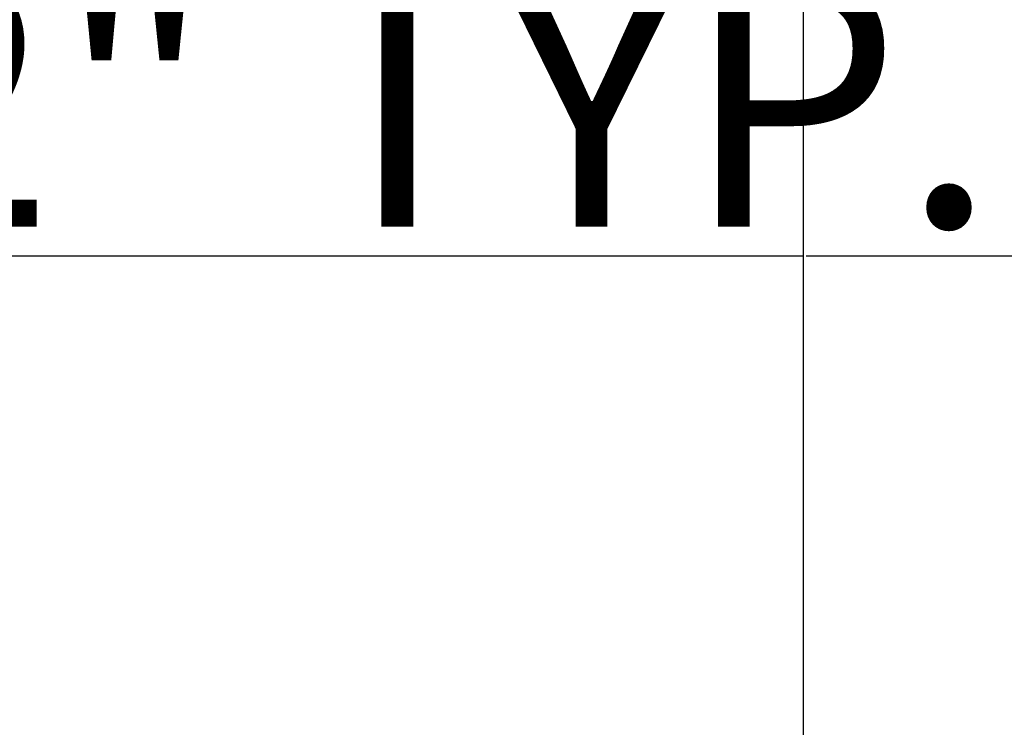
# Model space of a CAD drawing. Units: inches. Extents: x 2278 to 7495, y -71 to 1198.
# Tile 29 of 44: x 5127 to 5150, y 107 to 124. Entities that reach past the tile are written whole.
import ezdxf

# ---------------------------------------------------------------- set-up
doc = ezdxf.new("R2010")
doc.units = ezdxf.units.IN
doc.header["$MEASUREMENT"] = 0
doc.layers.add('A-ANNO-DIMS', color=2, linetype='Continuous', lineweight=18)
doc.layers.add('A-ELEV', color=7, linetype='Continuous', lineweight=25)
doc.styles.get("Standard").update_dxf_attribs({"font": 'arial.ttf'})
doc.dimstyles.get("Standard").update_dxf_attribs({"dimtxt": 6, "dimasz": 3, "dimexe": 0.18, "dimexo": 0.0625, "dimgap": 0.09, "dimtad": 0, "dimtih": 1, "dimtoh": 1, "dimdec": 0, "dimzin": 0, "dimdsep": 46, "dimlunit": 3, "dimtxsty": 'Standard', "dimblk": 'ARCHTICK', "dimcen": 0.09, "dimadec": 0, "dimazin": 0, "dimtfac": 1, "dimtdec": 0, "dimtofl": 0, "dimtmove": 0, "dimatfit": 3, "dimfxl": 1, "dimtolj": 1, "dimtzin": 0, "dimarcsym": 0})

# ---------------------------------------------------------------- blocks, each defined once
blk = doc.blocks.new('_ArchTick')
at = {"color": 0, "linetype": 'ByBlock', "const_width": 0.15}
blk.add_lwpolyline([(-0.5, -0.5), (0.5, 0.5)], dxfattribs=at)
blk = doc.blocks.new('*D59')
at = {"layer": 'A-ANNO-DIMS', "color": 0, "lineweight": -2, "transparency": 16777216}
for p, q in [((5096.589, 159.183), (5101.564, 159.183)), ((5101.384, 159.183), (5101.384, 146.185)), ((5101.384, 126.799), (5101.384, 139.796)), ((5096.589, 126.799), (5101.564, 126.799))]:
    blk.add_line(p, q, dxfattribs=at)
at = {"layer": 'Defpoints', "color": 0, "transparency": 16777216}
for p in [(5096.527, 159.183), (5101.384, 159.183), (5096.527, 126.799)]:
    blk.add_point(p, dxfattribs=at)
at = {"layer": 'A-ANNO-DIMS', "color": 0, "lineweight": -2, "transparency": 16777216, "xscale": 3, "yscale": 3, "zscale": 3}
for p, rotation in [((5101.384, 159.183), 90), ((5101.384, 126.799), 270)]:
    blk.add_blockref('_ArchTick', p, dxfattribs=dict(at, rotation=rotation))
at = {"layer": 'A-ANNO-DIMS', "color": 0, "transparency": 16777216, "insert": (5101.384, 142.991), "char_height": 6, "attachment_point": 5}
blk.add_mtext('\\A1;ORNATE BALUSTER 2\'-8 1/2" TYP.', dxfattribs=at)
blk = doc.blocks.new('*D60')
at = {"layer": 'A-ANNO-DIMS', "color": 0, "lineweight": -2, "transparency": 16777216}
for p, q in [((5088.787, 126.736), (5088.787, 121.761)), ((5096.527, 126.736), (5096.527, 121.761)), ((5088.787, 121.941), (5096.527, 121.941)), ((5096.527, 121.941), (5099.527, 121.941))]:
    blk.add_line(p, q, dxfattribs=at)
at = {"layer": 'Defpoints', "color": 0, "transparency": 16777216}
for p in [(5088.787, 126.799), (5096.527, 126.799), (5096.527, 121.941)]:
    blk.add_point(p, dxfattribs=at)
at = {"layer": 'A-ANNO-DIMS', "color": 0, "lineweight": -2, "transparency": 16777216, "xscale": 3, "yscale": 3, "zscale": 3, "rotation": 180}
blk.add_blockref('_ArchTick', (5088.787, 121.941), dxfattribs=at)
at = {"layer": 'A-ANNO-DIMS', "color": 0, "lineweight": -2, "transparency": 16777216, "xscale": 3, "yscale": 3, "zscale": 3}
blk.add_blockref('_ArchTick', (5096.527, 121.941), dxfattribs=at)
at = {"layer": 'A-ANNO-DIMS', "color": 0, "transparency": 16777216, "insert": (5124.894, 121.941), "char_height": 6, "attachment_point": 5}
blk.add_mtext('\\A1;0\'-7 1/2" TYP.', dxfattribs=at)
blk = doc.blocks.new('*D123')
at = {"layer": 'A-ANNO-DIMS', "color": 0, "lineweight": -2, "transparency": 16777216}
for p, q in [((4736.95, 340.157), (4736.95, -23.427)), ((5145.676, -1.81), (5145.676, -23.427)), ((4736.95, -23.247), (4923.929, -23.247)), ((5145.676, -23.247), (4958.697, -23.247))]:
    blk.add_line(p, q, dxfattribs=at)
at = {"layer": 'Defpoints', "color": 0, "transparency": 16777216}
for p in [(4736.95, 340.219), (5145.676, -1.747), (5145.676, -23.247)]:
    blk.add_point(p, dxfattribs=at)
at = {"layer": 'A-ANNO-DIMS', "color": 0, "lineweight": -2, "transparency": 16777216, "xscale": 3, "yscale": 3, "zscale": 3, "rotation": 180}
blk.add_blockref('_ArchTick', (4736.95, -23.247), dxfattribs=at)
at = {"layer": 'A-ANNO-DIMS', "color": 0, "lineweight": -2, "transparency": 16777216, "xscale": 3, "yscale": 3, "zscale": 3}
blk.add_blockref('_ArchTick', (5145.676, -23.247), dxfattribs=at)
at = {"layer": 'A-ANNO-DIMS', "color": 0, "transparency": 16777216, "insert": (4941.313, -23.247), "char_height": 6, "attachment_point": 5}
blk.add_mtext('\\A1;34\'-0 1/2"', dxfattribs=at)
blk = doc.blocks.new('*D131')
at = {"layer": 'A-ANNO-DIMS', "color": 0, "lineweight": -2, "transparency": 16777216}
for p, q in [((5096.176, 99.315), (5096.176, 361.899)), ((5145.676, 118.315), (5145.676, 361.899)), ((5096.176, 361.719), (5105.75, 361.719)), ((5145.676, 361.719), (5136.102, 361.719))]:
    blk.add_line(p, q, dxfattribs=at)
at = {"layer": 'Defpoints', "color": 0, "transparency": 16777216}
for p in [(5145.676, 361.719), (5145.676, 118.253), (5096.176, 99.253)]:
    blk.add_point(p, dxfattribs=at)
at = {"layer": 'A-ANNO-DIMS', "color": 0, "lineweight": -2, "transparency": 16777216, "xscale": 3, "yscale": 3, "zscale": 3, "rotation": 180}
blk.add_blockref('_ArchTick', (5096.176, 361.719), dxfattribs=at)
at = {"layer": 'A-ANNO-DIMS', "color": 0, "lineweight": -2, "transparency": 16777216, "xscale": 3, "yscale": 3, "zscale": 3}
blk.add_blockref('_ArchTick', (5145.676, 361.719), dxfattribs=at)
at = {"layer": 'A-ANNO-DIMS', "color": 0, "transparency": 16777216, "insert": (5120.926, 361.719), "char_height": 6, "attachment_point": 5}
blk.add_mtext('\\A1;4\'-1 1/2"', dxfattribs=at)
blk = doc.blocks.new('*D138')
at = {"layer": 'A-ANNO-DIMS', "color": 0, "lineweight": -2, "transparency": 16777216}
for p, q in [((5145.739, 118.253), (5167.754, 118.253)), ((5167.574, 118.253), (5167.574, 111.855)), ((5167.574, 99.253), (5167.574, 105.651)), ((5096.239, 99.253), (5167.754, 99.253))]:
    blk.add_line(p, q, dxfattribs=at)
at = {"layer": 'Defpoints', "color": 0, "transparency": 16777216}
for p in [(5145.676, 118.253), (5167.574, 118.253), (5096.176, 99.253)]:
    blk.add_point(p, dxfattribs=at)
at = {"layer": 'A-ANNO-DIMS', "color": 0, "lineweight": -2, "transparency": 16777216, "xscale": 3, "yscale": 3, "zscale": 3}
for p, rotation in [((5167.574, 118.253), 90), ((5167.574, 99.253), 270)]:
    blk.add_blockref('_ArchTick', p, dxfattribs=dict(at, rotation=rotation))
at = {"layer": 'A-ANNO-DIMS', "color": 0, "transparency": 16777216, "insert": (5167.574, 108.753), "char_height": 6, "attachment_point": 5}
blk.add_mtext('\\A1;1\'-7"', dxfattribs=at)
blk = doc.blocks.new('*D139')
at = {"layer": 'A-ANNO-DIMS', "color": 0, "lineweight": -2, "transparency": 16777216}
for p, q in [((5092.239, 160.253), (5167.754, 160.253)), ((5167.574, 160.253), (5167.574, 142.408)), ((5167.574, 118.253), (5167.574, 136.097)), ((5145.739, 118.253), (5167.754, 118.253))]:
    blk.add_line(p, q, dxfattribs=at)
at = {"layer": 'Defpoints', "color": 0, "transparency": 16777216}
for p in [(5092.176, 160.253), (5167.574, 160.253), (5145.676, 118.253)]:
    blk.add_point(p, dxfattribs=at)
at = {"layer": 'A-ANNO-DIMS', "color": 0, "lineweight": -2, "transparency": 16777216, "xscale": 3, "yscale": 3, "zscale": 3}
for p, rotation in [((5167.574, 160.253), 90), ((5167.574, 118.253), 270)]:
    blk.add_blockref('_ArchTick', p, dxfattribs=dict(at, rotation=rotation))
at = {"layer": 'A-ANNO-DIMS', "color": 0, "transparency": 16777216, "insert": (5167.574, 139.253), "char_height": 6, "attachment_point": 5}
blk.add_mtext('\\A1;3\'-6"', dxfattribs=at)
blk = doc.blocks.new('*D143')
at = {"layer": 'A-ANNO-DIMS', "color": 0, "lineweight": -2, "transparency": 16777216}
for p, q in [((5145.739, 118.253), (5167.754, 118.253)), ((5167.574, 118.253), (5167.574, 61.406)), ((5167.574, -1.747), (5167.574, 55.099)), ((5145.739, -1.747), (5167.754, -1.747))]:
    blk.add_line(p, q, dxfattribs=at)
at = {"layer": 'Defpoints', "color": 0, "transparency": 16777216}
for p in [(5145.676, 118.253), (5167.574, 118.253), (5145.676, -1.747)]:
    blk.add_point(p, dxfattribs=at)
at = {"layer": 'A-ANNO-DIMS', "color": 0, "lineweight": -2, "transparency": 16777216, "xscale": 3, "yscale": 3, "zscale": 3}
for p, rotation in [((5167.574, 118.253), 90), ((5167.574, -1.747), 270)]:
    blk.add_blockref('_ArchTick', p, dxfattribs=dict(at, rotation=rotation))
at = {"layer": 'A-ANNO-DIMS', "color": 0, "transparency": 16777216, "insert": (5167.574, 58.253), "char_height": 6, "attachment_point": 5}
blk.add_mtext('\\A1;10\'-0"', dxfattribs=at)
blk = doc.blocks.new('*D144')
at = {"layer": 'A-ANNO-DIMS', "color": 0, "lineweight": -2, "transparency": 16777216}
for p, q in [((5145.739, 244.253), (5167.754, 244.253)), ((5167.574, 244.253), (5167.574, 184.406)), ((5167.574, 118.253), (5167.574, 178.099)), ((5145.739, 118.253), (5167.754, 118.253))]:
    blk.add_line(p, q, dxfattribs=at)
at = {"layer": 'Defpoints', "color": 0, "transparency": 16777216}
for p in [(5145.676, 244.253), (5167.574, 244.253), (5145.676, 118.253)]:
    blk.add_point(p, dxfattribs=at)
at = {"layer": 'A-ANNO-DIMS', "color": 0, "lineweight": -2, "transparency": 16777216, "xscale": 3, "yscale": 3, "zscale": 3}
for p, rotation in [((5167.574, 244.253), 90), ((5167.574, 118.253), 270)]:
    blk.add_blockref('_ArchTick', p, dxfattribs=dict(at, rotation=rotation))
at = {"layer": 'A-ANNO-DIMS', "color": 0, "transparency": 16777216, "insert": (5167.574, 181.253), "char_height": 6, "attachment_point": 5}
blk.add_mtext('\\A1;10\'-6"', dxfattribs=at)

msp = doc.modelspace()

# ---------------------------------------------------------------- linework, layer by layer
at = {"layer": 'A-ELEV'}
for p, q in [((5145.676, -1.747), (5145.676, 161.577)), ((4874.676, 118.253), (5145.676, 118.253))]:
    msp.add_line(p, q, dxfattribs=at)

# ---------------------------------------------------------------- dimensions: what is measured, and where the dimension line sits
at = {"layer": 'A-ANNO-DIMS'}
for base, p1, p2, picture, middle in [((5145.676, 361.719), (5096.176, 99.253), (5145.676, 118.253), '*D131', (5120.926, 361.719)), ((5145.676, -23.247), (4736.95, 340.219), (5145.676, -1.747), '*D123', (4941.313, -23.247))]:
    dim = msp.add_linear_dim(base=base, p1=p1, p2=p2, dimstyle='Standard', override={"dimdec": 1, "dimlfac": 1, "dimrnd": 0, "dimzin": 1, "dimdsep": 46, "dimlunit": 4, "dimfrac": 2}, dxfattribs=at)
    dim.commit()
    dim.dimension.update_dxf_attribs({"geometry": picture, "text_midpoint": middle})
for base, p1, p2, picture, middle in [((5167.574, 244.253), (5145.676, 118.253), (5145.676, 244.253), '*D144', (5167.574, 181.253)), ((5167.574, 160.253), (5145.676, 118.253), (5092.176, 160.253), '*D139', (5167.574, 139.253)), ((5167.574, 118.253), (5096.176, 99.253), (5145.676, 118.253), '*D138', (5167.574, 108.753)), ((5167.574, 118.253), (5145.676, -1.747), (5145.676, 118.253), '*D143', (5167.574, 58.253))]:
    dim = msp.add_linear_dim(base=base, p1=p1, p2=p2, angle=90, dimstyle='Standard', override={"dimdec": 1, "dimlfac": 1, "dimrnd": 0, "dimzin": 1, "dimdsep": 46, "dimlunit": 4, "dimfrac": 2}, dxfattribs=at)
    dim.commit()
    dim.dimension.update_dxf_attribs({"geometry": picture, "text_midpoint": middle})
dim = msp.add_linear_dim(base=(5101.384, 159.183), p1=(5096.527, 126.799), p2=(5096.527, 159.183), angle=90, text='ORNATE BALUSTER <> TYP.', dimstyle='Standard', override={"dimdec": 1, "dimrnd": 0, "dimzin": 1, "dimlunit": 4, "dimfrac": 2}, dxfattribs=at)
dim.commit()
dim.dimension.update_dxf_attribs({"geometry": '*D59', "text_midpoint": (5101.384, 142.991)})
dim = msp.add_linear_dim(base=(5096.527, 121.941), p1=(5088.787, 126.799), p2=(5096.527, 126.799), text='<> TYP.', dimstyle='Standard', override={"dimdec": 1, "dimrnd": 0, "dimzin": 1, "dimlunit": 4, "dimfrac": 2}, dxfattribs=at)
dim.commit()
dim.dimension.update_dxf_attribs({"geometry": '*D60', "text_midpoint": (5124.894, 121.941)})

doc.saveas('drawing.dxf')
